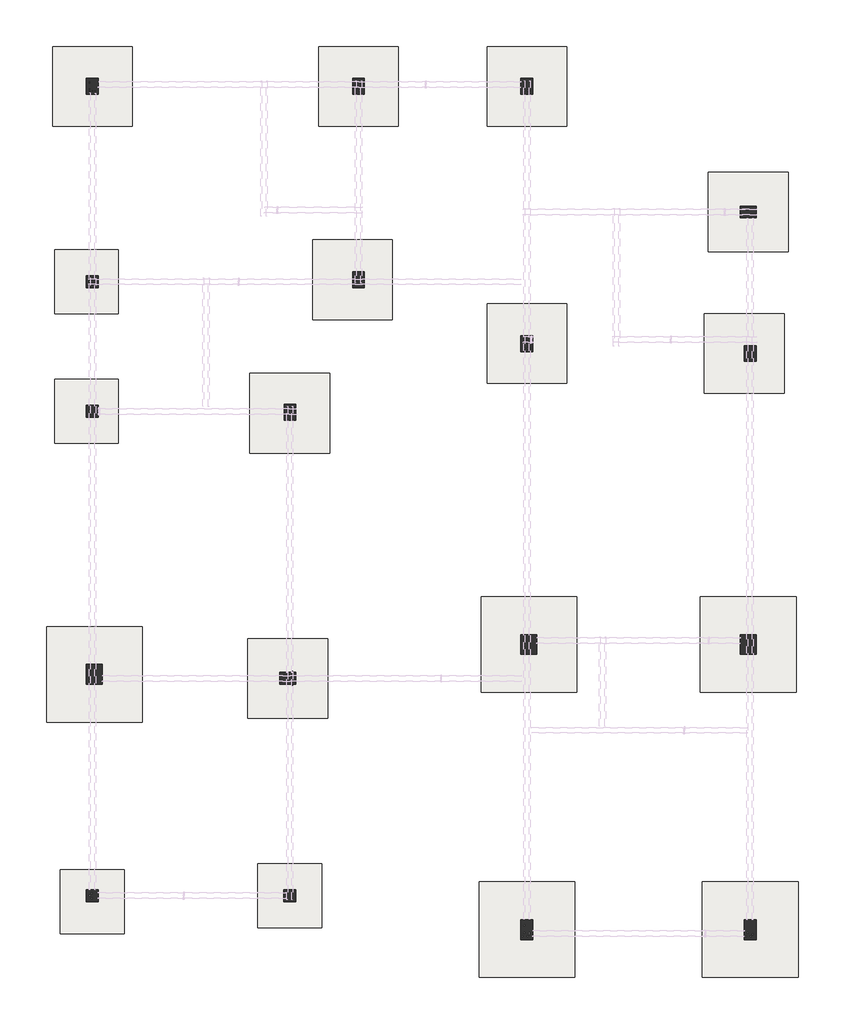
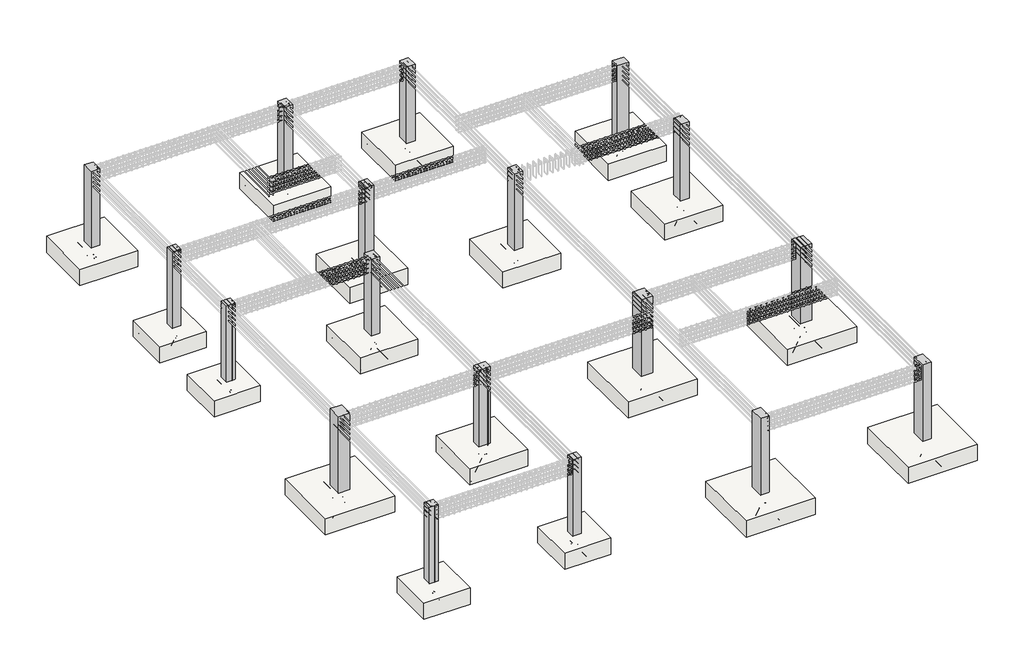
# One storey, part 1 of 10: 18 columns, 18 slabs.
"""IFC4 building model written with IfcOpenShell, lengths in millimetres."""

from ifc_helpers import new_model, si_unit, frame, origin, place, context, project, spatial, polyline, outline, extrude, faceted_brep, transform, mapped, element, save
from components import m_footing_rectangular_4_x4_72b13ef4, m_footing_rectangular_5_x5_4154a230, m_footing_rectangular_6_x6_603268f9

model = new_model("IFC4")

# Units and contexts
model_context = context("Model", 3, world=origin())
ifc_project = project(units=[si_unit("LENGTHUNIT", "METRE", prefix="MILLI")], contexts=[model_context])

# Site, building, storey
site = spatial("IfcSite", under=ifc_project)
building = spatial("IfcBuilding", under=site)
storey = spatial("IfcBuildingStorey", under=building, Elevation=-2133.6)

# Columns
placement = place(None, origin())
element("IfcColumn", 1, ObjectType="M_Concrete-Rectangular-Column : 12\" x 15\" c3", at=placement, inside=storey, context=model_context, shape_type="Brep", body=[
    faceted_brep([(-4744.7664362, 1101.7719177, -2133.6), (-4744.7664362, 720.7719177, -2133.6), (-5049.5664362, 720.7719177, -2133.6), (-5049.5664362, 1101.7719177, -2133.6), (-4744.7664362, 1101.7719177, 0.0), (-4744.7664362, 720.7719177, 0.0), (-4820.9664362, 720.7719177, 0.0), (-5049.5664362, 720.7719177, 0.0), (-5049.5664362, 720.7719177, -500.0), (-5049.5664362, 1101.7719177, 0.0), (-5049.5664362, 1101.7719177, -500.0), (-4820.9664362, 1101.7719177, 0.0)], [[[0, 1, 2, 3]], [[4, 5, 1, 0]], [[5, 6, 7, 8, 2, 1]], [[7, 9, 10, 3, 2, 8]], [[9, 11, 4, 0, 3, 10]], [[4, 11, 9, 7, 6, 5]]]),
])
element("IfcColumn", 2, ObjectType="M_Concrete-Rectangular-Column : 12\" x 15\" c3", at=placement, inside=storey, context=model_context, shape_type="Brep", body=[
    faceted_brep([(3561.0335638, 1674.0339177, -2133.6), (3561.0335638, 1293.0339177, -2133.6), (3256.2335638, 1293.0339177, -2133.6), (3256.2335638, 1674.0339177, -2133.6), (3561.0335638, 1674.0339177, 0.0), (3561.0335638, 1293.0339177, 0.0), (3484.8335638, 1293.0339177, 0.0), (3256.2335638, 1293.0339177, 0.0), (3256.2335638, 1293.0339177, -500.0), (3256.2335638, 1674.0339177, 0.0), (3256.2335638, 1674.0339177, -500.0), (3484.8335638, 1674.0339177, 0.0)], [[[0, 1, 2, 3]], [[4, 5, 1, 0]], [[5, 6, 7, 8, 2, 1]], [[7, 9, 10, 3, 2, 8]], [[9, 11, 4, 0, 3, 10]], [[4, 11, 9, 7, 6, 5]]]),
])
element("IfcColumn", 3, ObjectType="M_Concrete-Rectangular-Column : 12\" x 15\" c3", at=placement, inside=storey, context=model_context, shape_type="Brep", body=[
    faceted_brep([(7752.0335638, 1674.0339177, -2133.6), (7752.0335638, 1293.0339177, -2133.6), (7447.2335638, 1293.0339177, -2133.6), (7447.2335638, 1674.0339177, -2133.6), (7752.0335638, 1674.0339177, 0.0), (7752.0335638, 1293.0339177, 0.0), (7752.0335638, 1293.0339177, -500.0), (7752.0335638, 1674.0339177, -500.0), (7523.4335638, 1293.0339177, 0.0), (7447.2335638, 1293.0339177, 0.0), (7447.2335638, 1674.0339177, 0.0), (7523.4335638, 1674.0339177, 0.0)], [[[0, 1, 2, 3]], [[4, 5, 6, 1, 0, 7]], [[5, 8, 9, 2, 1, 6]], [[9, 10, 3, 2]], [[10, 11, 4, 7, 0, 3]], [[4, 11, 10, 9, 8, 5]]]),
])
element("IfcColumn", 4, ObjectType="M_Concrete-Rectangular-Column : 12\" x 9\" c4", at=placement, inside=storey, context=model_context, shape_type="Brep", body=[
    faceted_brep([(-1049.0664362, 949.3719177, -2133.6), (-1049.0664362, 720.7719177, -2133.6), (-1353.8664362, 720.7719177, -2133.6), (-1353.8664362, 949.3719177, -2133.6), (-1049.0664362, 949.3719177, 0.0), (-1049.0664362, 720.7719177, 0.0), (-1049.0664362, 720.7719177, -500.0), (-1049.0664362, 949.3719177, -500.0), (-1353.8664362, 720.7719177, 0.0), (-1353.8664362, 720.7719177, -500.0), (-1353.8664362, 949.3719177, 0.0), (-1353.8664362, 949.3719177, -500.0)], [[[0, 1, 2, 3]], [[4, 5, 6, 1, 0, 7]], [[5, 8, 9, 2, 1, 6]], [[8, 10, 11, 3, 2, 9]], [[10, 4, 7, 0, 3, 11]], [[4, 10, 8, 5]]]),
])
element("IfcColumn", 5, ObjectType="M_Concrete-Rectangular-Column : 9\" x 12\" c1", at=placement, inside=storey, context=model_context, shape_type="SweptSolid", body=[
    extrude(outline(polyline([(-4820.9664362, 12303.1719177), (-4820.9664362, 11998.3719177), (-5049.5664362, 11998.3719177), (-5049.5664362, 12303.1719177), (-4820.9664362, 12303.1719177)])), frame((0.0, 0.0, -2133.6), z_axis=(0.0, 0.0, 1.0), x_axis=(1.0, 0.0, 0.0)), (0.0, 0.0, 1.0), 2133.6),
])
element("IfcColumn", 6, ObjectType="M_Concrete-Rectangular-Column : 9\" x 12\" c1", at=placement, inside=storey, context=model_context, shape_type="Brep", body=[
    faceted_brep([(265.3835638, 12303.1719177, -2133.6), (265.3835638, 11998.3719177, -2133.6), (36.7835638, 11998.3719177, -2133.6), (36.7835638, 12303.1719177, -2133.6), (265.3835638, 12303.1719177, 0.0), (265.3835638, 12074.5719177, 0.0), (265.3835638, 11998.3719177, 0.0), (265.3835638, 12303.1719177, -500.0), (36.7835638, 11998.3719177, 0.0), (36.7835638, 12074.5719177, 0.0), (36.7835638, 12303.1719177, 0.0), (36.7835638, 12303.1719177, -500.0)], [[[0, 1, 2, 3]], [[4, 5, 6, 1, 0, 7]], [[6, 8, 2, 1]], [[8, 9, 10, 11, 3, 2]], [[10, 4, 7, 0, 3, 11]], [[4, 10, 9, 8, 6, 5]]]),
])
element("IfcColumn", 7, ObjectType="M_Concrete-Rectangular-Column : 9\" x 12\" c1", at=placement, inside=storey, context=model_context, shape_type="SweptSolid", body=[
    extrude(outline(polyline([(3484.8335638, 12303.1719177), (3484.8335638, 11998.3719177), (3256.2335638, 11998.3719177), (3256.2335638, 12303.1719177), (3484.8335638, 12303.1719177)])), frame((0.0, 0.0, -2133.6), z_axis=(0.0, 0.0, 1.0), x_axis=(1.0, 0.0, 0.0)), (0.0, 0.0, 1.0), 2133.6),
])
element("IfcColumn", 8, ObjectType="M_Concrete-Rectangular-Column : 9\" x 12\" c1", at=placement, inside=storey, context=model_context, shape_type="Brep", body=[
    faceted_brep([(265.3835638, 8607.4719177, -2133.6), (265.3835638, 8302.6719177, -2133.6), (36.7835638, 8302.6719177, -2133.6), (36.7835638, 8607.4719177, -2133.6), (265.3835638, 8607.4719177, 0.0), (265.3835638, 8531.2719177, 0.0), (265.3835638, 8302.6719177, 0.0), (265.3835638, 8302.6719177, -500.0), (36.7835638, 8302.6719177, 0.0), (36.7835638, 8302.6719177, -500.0), (36.7835638, 8531.2719177, 0.0), (36.7835638, 8607.4719177, 0.0)], [[[0, 1, 2, 3]], [[4, 5, 6, 7, 1, 0]], [[6, 8, 9, 2, 1, 7]], [[8, 10, 11, 3, 2, 9]], [[11, 4, 0, 3]], [[4, 11, 10, 8, 6, 5]]]),
])
element("IfcColumn", 9, ObjectType="M_Concrete-Rectangular-Column : 9\" x 12\" c1", at=placement, inside=storey, context=model_context, shape_type="SweptSolid", body=[
    extrude(outline(polyline([(-1043.9664362, 6072.8719177), (-1043.9664362, 5768.0719177), (-1272.5664362, 5768.0719177), (-1272.5664362, 6072.8719177), (-1043.9664362, 6072.8719177)])), frame((0.0, 0.0, -2133.6), z_axis=(0.0, 0.0, 1.0), x_axis=(1.0, 0.0, 0.0)), (0.0, 0.0, 1.0), 2133.6),
])
element("IfcColumn", 10, ObjectType="M_Concrete-Rectangular-Column : 9\" x 12\" c1", at=placement, inside=storey, context=model_context, shape_type="Brep", body=[
    faceted_brep([(3484.8335638, 7388.2719177, -2133.6), (3484.8335638, 7083.4719177, -2133.6), (3256.2335638, 7083.4719177, -2133.6), (3256.2335638, 7388.2719177, -2133.6), (3484.8335638, 7388.2719177, 0.0), (3484.8335638, 7197.7719177, 0.0), (3484.8335638, 7083.4719177, 0.0), (3484.8335638, 7083.4719177, -500.0), (3484.8335638, 7388.2719177, -500.0), (3256.2335638, 7083.4719177, 0.0), (3256.2335638, 7083.4719177, -500.0), (3256.2335638, 7388.2719177, 0.0), (3256.2335638, 7388.2719177, -500.0)], [[[0, 1, 2, 3]], [[4, 5, 6, 7, 1, 0, 8]], [[6, 9, 10, 2, 1, 7]], [[9, 11, 12, 3, 2, 10]], [[11, 4, 8, 0, 3, 12]], [[4, 11, 9, 6, 5]]]),
])
element("IfcColumn", 11, ObjectType="M_Concrete-Rectangular-Column : 9\" x 12\" c1", at=placement, inside=storey, context=model_context, shape_type="SweptSolid", body=[
    extrude(outline(polyline([(7447.2335638, 9864.7719177), (7752.0335638, 9864.7719177), (7752.0335638, 9636.1719177), (7447.2335638, 9636.1719177), (7447.2335638, 9864.7719177)])), frame((0.0, 0.0, -2133.6), z_axis=(0.0, 0.0, 1.0), x_axis=(1.0, 0.0, 0.0)), (0.0, 0.0, 1.0), 2133.6),
])
element("IfcColumn", 12, ObjectType="M_Concrete-Rectangular-Column : 9\" x 12\" c1", at=placement, inside=storey, context=model_context, shape_type="Brep", body=[
    faceted_brep([(7752.0335638, 7197.7719177, -2133.6), (7752.0335638, 6892.9719177, -2133.6), (7523.4335638, 6892.9719177, -2133.6), (7523.4335638, 7197.7719177, -2133.6), (7752.0335638, 7197.7719177, 0.0), (7752.0335638, 6892.9719177, 0.0), (7752.0335638, 6892.9719177, -500.0), (7752.0335638, 7197.7719177, -500.0), (7523.4335638, 6892.9719177, 0.0), (7523.4335638, 6892.9719177, -500.0), (7523.4335638, 7197.7719177, 0.0), (7523.4335638, 7197.7719177, -500.0)], [[[0, 1, 2, 3]], [[4, 5, 6, 1, 0, 7]], [[5, 8, 9, 2, 1, 6]], [[8, 10, 11, 3, 2, 9]], [[10, 4, 7, 0, 3, 11]], [[4, 10, 8, 5]]]),
])
element("IfcColumn", 13, ObjectType="M_Concrete-Rectangular-Column : 9\" x 15\" c5", at=placement, inside=storey, context=model_context, shape_type="SweptSolid", body=[
    extrude(outline(polyline([(3484.8335638, -3775.0280823), (3484.8335638, -4156.0280823), (3256.2335638, -4156.0280823), (3256.2335638, -3775.0280823), (3484.8335638, -3775.0280823)])), frame((0.0, 0.0, -2133.6), z_axis=(0.0, 0.0, 1.0), x_axis=(1.0, 0.0, 0.0)), (0.0, 0.0, 1.0), 2133.6),
])
element("IfcColumn", 14, ObjectType="M_Concrete-Rectangular-Column : 9\" x 15\" c5", at=placement, inside=storey, context=model_context, shape_type="SweptSolid", body=[
    extrude(outline(polyline([(7752.0335638, -3775.0280823), (7752.0335638, -4156.0280823), (7523.4335638, -4156.0280823), (7523.4335638, -3775.0280823), (7752.0335638, -3775.0280823)])), frame((0.0, 0.0, -2133.6), z_axis=(0.0, 0.0, 1.0), x_axis=(1.0, 0.0, 0.0)), (0.0, 0.0, 1.0), 2133.6),
])
element("IfcColumn", 15, ObjectType="M_Concrete-Rectangular-Column : 9\" x9\" c2", at=placement, inside=storey, context=model_context, shape_type="Brep", body=[
    faceted_brep([(-4820.9664362, 8531.2719177, -2133.6), (-4820.9664362, 8302.6719177, -2133.6), (-5049.5664362, 8302.6719177, -2133.6), (-5049.5664362, 8531.2719177, -2133.6), (-4820.9664362, 8531.2719177, 0.0), (-4820.9664362, 8302.6719177, 0.0), (-4820.9664362, 8302.6719177, -500.0), (-4820.9664362, 8531.2719177, -500.0), (-5049.5664362, 8302.6719177, 0.0), (-5049.5664362, 8302.6719177, -500.0), (-5049.5664362, 8531.2719177, 0.0), (-5049.5664362, 8531.2719177, -500.0)], [[[0, 1, 2, 3]], [[4, 5, 6, 1, 0, 7]], [[5, 8, 9, 2, 1, 6]], [[8, 10, 11, 3, 2, 9]], [[10, 4, 7, 0, 3, 11]], [[4, 10, 8, 5]]]),
])
element("IfcColumn", 16, ObjectType="M_Concrete-Rectangular-Column : 9\" x9\" c2", at=placement, inside=storey, context=model_context, shape_type="Brep", body=[
    faceted_brep([(-4820.9664362, 6054.7719177, -2133.6), (-4820.9664362, 5826.1719177, -2133.6), (-5049.5664362, 5826.1719177, -2133.6), (-5049.5664362, 6054.7719177, -2133.6), (-4820.9664362, 6054.7719177, 0.0), (-4820.9664362, 5826.1719177, 0.0), (-4820.9664362, 5826.1719177, -500.0), (-4820.9664362, 6054.7719177, -500.0), (-5049.5664362, 5826.1719177, 0.0), (-5049.5664362, 5826.1719177, -500.0), (-5049.5664362, 6054.7719177, 0.0), (-5049.5664362, 6054.7719177, -500.0)], [[[0, 1, 2, 3]], [[4, 5, 6, 1, 0, 7]], [[5, 8, 9, 2, 1, 6]], [[8, 10, 11, 3, 2, 9]], [[10, 4, 7, 0, 3, 11]], [[4, 10, 8, 5]]]),
])
element("IfcColumn", 17, ObjectType="M_Concrete-Rectangular-Column : 9\" x9\" c2", at=placement, inside=storey, context=model_context, shape_type="SweptSolid", body=[
    extrude(outline(polyline([(-4820.9664362, -3203.5280823), (-4820.9664362, -3432.1280823), (-5049.5664362, -3432.1280823), (-5049.5664362, -3203.5280823), (-4820.9664362, -3203.5280823)])), frame((0.0, 0.0, -2133.6), z_axis=(0.0, 0.0, 1.0), x_axis=(1.0, 0.0, 0.0)), (0.0, 0.0, 1.0), 2133.6),
])
element("IfcColumn", 18, ObjectType="M_Concrete-Rectangular-Column : 9\" x9\" c2", at=placement, inside=storey, context=model_context, shape_type="SweptSolid", body=[
    extrude(outline(polyline([(-1049.0664362, -3203.5280823), (-1049.0664362, -3432.1280823), (-1277.6664362, -3432.1280823), (-1277.6664362, -3203.5280823), (-1049.0664362, -3203.5280823)])), frame((0.0, 0.0, -2133.6), z_axis=(0.0, 0.0, 1.0), x_axis=(1.0, 0.0, 0.0)), (0.0, 0.0, 1.0), 2133.6),
])

# Slabs
m_footing_rectangular_4_x4_shape = m_footing_rectangular_4_x4_72b13ef4(model_context)
element("IfcSlab", 19, ObjectType="M_Footing-Rectangular : 4'x4'", at=placement, inside=storey, context=model_context, shape_type="MappedRepresentation", body=[
    mapped(m_footing_rectangular_4_x4_shape, transform((-5049.5664362, 8416.9719177, -2133.6), x_axis=(1.0, 0.0, 0.0), y_axis=(0.0, 1.0, 0.0), z_axis=(0.0, 0.0, 1.0))),
])
element("IfcSlab", 20, ObjectType="M_Footing-Rectangular : 4'x4'", at=placement, inside=storey, context=model_context, shape_type="MappedRepresentation", body=[
    mapped(m_footing_rectangular_4_x4_shape, transform((-5049.5664362, 5940.4719177, -2133.6), x_axis=(1.0, 0.0, 0.0), y_axis=(0.0, 1.0, 0.0), z_axis=(0.0, 0.0, 1.0))),
])
element("IfcSlab", 21, ObjectType="M_Footing-Rectangular : 4'x4'", at=placement, inside=storey, context=model_context, shape_type="MappedRepresentation", body=[
    mapped(m_footing_rectangular_4_x4_shape, transform((-4935.2664362, -3432.1280823, -2133.6), x_axis=(1.0, 0.0, 0.0), y_axis=(0.0, 1.0, 0.0), z_axis=(0.0, 0.0, 1.0))),
])
element("IfcSlab", 22, ObjectType="M_Footing-Rectangular : 4'x4'", at=placement, inside=storey, context=model_context, shape_type="MappedRepresentation", body=[
    mapped(m_footing_rectangular_4_x4_shape, transform((-1163.3664362, -3317.8280823, -2133.6), x_axis=(1.0, 0.0, 0.0), y_axis=(0.0, 1.0, 0.0), z_axis=(0.0, 0.0, 1.0))),
])
m_footing_rectangular_5_x5_shape = m_footing_rectangular_5_x5_4154a230(model_context)
element("IfcSlab", 23, ObjectType="M_Footing-Rectangular : 5'x5'", at=placement, inside=storey, context=model_context, shape_type="MappedRepresentation", body=[
    mapped(m_footing_rectangular_5_x5_shape, transform((-4935.2664362, 12150.7719177, -2133.6), x_axis=(1.0, 0.0, 0.0), y_axis=(0.0, 1.0, 0.0), z_axis=(0.0, 0.0, 1.0))),
])
element("IfcSlab", 24, ObjectType="M_Footing-Rectangular : 5'x5'", at=placement, inside=storey, context=model_context, shape_type="MappedRepresentation", body=[
    mapped(m_footing_rectangular_5_x5_shape, transform((151.0835638, 12150.7719177, -2133.6), x_axis=(1.0, 0.0, 0.0), y_axis=(0.0, 1.0, 0.0), z_axis=(0.0, 0.0, 1.0))),
])
element("IfcSlab", 25, ObjectType="M_Footing-Rectangular : 5'x5'", at=placement, inside=storey, context=model_context, shape_type="MappedRepresentation", body=[
    mapped(m_footing_rectangular_5_x5_shape, transform((3370.5335638, 12150.7719177, -2133.6), x_axis=(1.0, 0.0, 0.0), y_axis=(0.0, 1.0, 0.0), z_axis=(0.0, 0.0, 1.0))),
])
element("IfcSlab", 26, ObjectType="M_Footing-Rectangular : 5'x5'", at=placement, inside=storey, context=model_context, shape_type="MappedRepresentation", body=[
    mapped(m_footing_rectangular_5_x5_shape, transform((7599.6335638, 9750.4719177, -2133.6), x_axis=(1.0, 0.0, 0.0), y_axis=(0.0, 1.0, 0.0), z_axis=(0.0, 0.0, 1.0))),
])
element("IfcSlab", 27, ObjectType="M_Footing-Rectangular : 5'x5'", at=placement, inside=storey, context=model_context, shape_type="MappedRepresentation", body=[
    mapped(m_footing_rectangular_5_x5_shape, transform((36.7835638, 8455.0719177, -2133.6), x_axis=(1.0, 0.0, 0.0), y_axis=(0.0, 1.0, 0.0), z_axis=(0.0, 0.0, 1.0))),
])
element("IfcSlab", 28, ObjectType="M_Footing-Rectangular : 5'x5'", at=placement, inside=storey, context=model_context, shape_type="MappedRepresentation", body=[
    mapped(m_footing_rectangular_5_x5_shape, transform((7523.4335638, 7045.3719177, -2133.6), x_axis=(1.0, 0.0, 0.0), y_axis=(0.0, 1.0, 0.0), z_axis=(0.0, 0.0, 1.0))),
])
element("IfcSlab", 29, ObjectType="M_Footing-Rectangular : 5'x5'", at=placement, inside=storey, context=model_context, shape_type="MappedRepresentation", body=[
    mapped(m_footing_rectangular_5_x5_shape, transform((3370.5335638, 7235.8719177, -2133.6), x_axis=(1.0, 0.0, 0.0), y_axis=(0.0, 1.0, 0.0), z_axis=(0.0, 0.0, 1.0))),
])
element("IfcSlab", 30, ObjectType="M_Footing-Rectangular : 5'x5'", at=placement, inside=storey, context=model_context, shape_type="MappedRepresentation", body=[
    mapped(m_footing_rectangular_5_x5_shape, transform((-1163.3664362, 5902.3719177, -2133.6), x_axis=(1.0, 0.0, 0.0), y_axis=(0.0, 1.0, 0.0), z_axis=(0.0, 0.0, 1.0))),
])
element("IfcSlab", 31, ObjectType="M_Footing-Rectangular : 5'x5'", at=placement, inside=storey, context=model_context, shape_type="MappedRepresentation", body=[
    mapped(m_footing_rectangular_5_x5_shape, transform((-1201.4664362, 835.0719177, -2133.6), x_axis=(1.0, 0.0, 0.0), y_axis=(0.0, 1.0, 0.0), z_axis=(0.0, 0.0, 1.0))),
])
m_footing_rectangular_6_x6_shape = m_footing_rectangular_6_x6_603268f9(model_context)
element("IfcSlab", 32, ObjectType="M_Footing-Rectangular : 6' x6'", at=placement, inside=storey, context=model_context, shape_type="MappedRepresentation", body=[
    mapped(m_footing_rectangular_6_x6_shape, transform((-4897.1664362, 911.2719177, -2133.6), x_axis=(1.0, 0.0, 0.0), y_axis=(0.0, 1.0, 0.0), z_axis=(0.0, 0.0, 1.0))),
])
element("IfcSlab", 33, ObjectType="M_Footing-Rectangular : 6' x6'", at=placement, inside=storey, context=model_context, shape_type="MappedRepresentation", body=[
    mapped(m_footing_rectangular_6_x6_shape, transform((3408.6335638, 1483.5339177, -2133.6), x_axis=(1.0, 0.0, 0.0), y_axis=(0.0, 1.0, 0.0), z_axis=(0.0, 0.0, 1.0))),
])
element("IfcSlab", 34, ObjectType="M_Footing-Rectangular : 6' x6'", at=placement, inside=storey, context=model_context, shape_type="MappedRepresentation", body=[
    mapped(m_footing_rectangular_6_x6_shape, transform((7599.6335638, 1483.5339177, -2133.6), x_axis=(1.0, 0.0, 0.0), y_axis=(0.0, 1.0, 0.0), z_axis=(0.0, 0.0, 1.0))),
])
element("IfcSlab", 35, ObjectType="M_Footing-Rectangular : 6' x6'", at=placement, inside=storey, context=model_context, shape_type="MappedRepresentation", body=[
    mapped(m_footing_rectangular_6_x6_shape, transform((7637.7335638, -3965.5280823, -2133.6), x_axis=(1.0, 0.0, 0.0), y_axis=(0.0, 1.0, 0.0), z_axis=(0.0, 0.0, 1.0))),
])
element("IfcSlab", 36, ObjectType="M_Footing-Rectangular : 6' x6'", at=placement, inside=storey, context=model_context, shape_type="MappedRepresentation", body=[
    mapped(m_footing_rectangular_6_x6_shape, transform((3370.5335638, -3965.5280823, -2133.6), x_axis=(1.0, 0.0, 0.0), y_axis=(0.0, 1.0, 0.0), z_axis=(0.0, 0.0, 1.0))),
])

save(model, "model.ifc")

# Revit data of these elements
# Type "M_Concrete-Rectangular-Column : 12\" x 15\" c3"
#   b = 1' - 0"
#   h = 1' - 3"
#   Structural Material [instance default] = Concrete, Cast-in-Place gray
# Type "M_Concrete-Rectangular-Column : 12\" x 9\" c4"
#   b = 1' - 0"
#   h = 0' - 9"
#   Structural Material [instance default] = Concrete, Cast-in-Place gray
# Type "M_Concrete-Rectangular-Column : 9\" x 12\" c1"
#   b = 0' - 9"
#   h = 1' - 0"
#   Structural Material [instance default] = Concrete, Cast-in-Place gray
# Type "M_Concrete-Rectangular-Column : 9\" x 15\" c5"
#   b = 0' - 9"
#   h = 1' - 3"
#   Structural Material [instance default] = Concrete, Cast-in-Place gray
# Type "M_Concrete-Rectangular-Column : 9\" x9\" c2"
#   b = 0' - 9"
#   h = 0' - 9"
#   Structural Material [instance default] = Concrete, Cast-in-Place gray
# Type "M_Footing-Rectangular : 4'x4'"
#   Width = 4' - 0"
#   Length = 4' - 0"
#   Foundation Thickness = 1' - 5.71654"
#   Structural Material [instance default] = Concrete, Cast-in-Place gray
#   Assembly Code = ""
# Type "M_Footing-Rectangular : 5'x5'"
#   Width = 5' - 0"
#   Length = 5' - 0"
#   Foundation Thickness = 1' - 5.71654"
#   Structural Material [instance default] = Concrete, Cast-in-Place gray
#   Assembly Code = ""
# Type "M_Footing-Rectangular : 6' x6'"
#   Width = 6' - 0"
#   Length = 6' - 0"
#   Foundation Thickness = 1' - 5.71654"
#   Structural Material [instance default] = Concrete, Cast-in-Place gray
#   Assembly Code = ""
# Elements 1, 2, 3 (IfcColumn, "M_Concrete-Rectangular-Column : 12\" x 15\" c3")
#   Structural Material = Concrete, Cast-in-Place gray
#   Phase Created = New Construction
#   Materials on its faces: "Concrete, Cast-in-Place gray"
# Element 4 (IfcColumn, "M_Concrete-Rectangular-Column : 12\" x 9\" c4")
#   Structural Material = Concrete, Cast-in-Place gray
#   Phase Created = New Construction
#   Materials on its faces: "Concrete, Cast-in-Place gray"
# Elements 5, 6, 7, 8, 9, 10, 11, 12 (IfcColumn, "M_Concrete-Rectangular-Column : 9\" x 12\" c1")
#   Structural Material = Concrete, Cast-in-Place gray
#   Phase Created = New Construction
#   Materials on its faces: "Concrete, Cast-in-Place gray"
# Elements 13, 14 (IfcColumn, "M_Concrete-Rectangular-Column : 9\" x 15\" c5")
#   Structural Material = Concrete, Cast-in-Place gray
#   Phase Created = New Construction
#   Materials on its faces: "Concrete, Cast-in-Place gray"
# Elements 15, 16, 17, 18 (IfcColumn, "M_Concrete-Rectangular-Column : 9\" x9\" c2")
#   Structural Material = Concrete, Cast-in-Place gray
#   Phase Created = New Construction
#   Materials on its faces: "Concrete, Cast-in-Place gray"
# Elements 19, 20, 21, 22 (IfcSlab, "M_Footing-Rectangular : 4'x4'")
#   Structural Material = Concrete, Cast-in-Place gray
#   Phase Created = New Construction
#   Materials on its faces: "Concrete, Cast-in-Place gray"
# Elements 23, 24, 25, 26, 27, 28, 29, 30, 31 (IfcSlab, "M_Footing-Rectangular : 5'x5'")
#   Structural Material = Concrete, Cast-in-Place gray
#   Phase Created = New Construction
#   Materials on its faces: "Concrete, Cast-in-Place gray"
# Elements 32, 33, 34, 35, 36 (IfcSlab, "M_Footing-Rectangular : 6' x6'")
#   Structural Material = Concrete, Cast-in-Place gray
#   Phase Created = New Construction
#   Materials on its faces: "Concrete, Cast-in-Place gray"
# Materials
#   "Concrete, Cast-in-Place gray": class "Concrete", colour RGB 192 192 192, transparency 0, Description = "Cast-in-place concrete", Cost = 0
